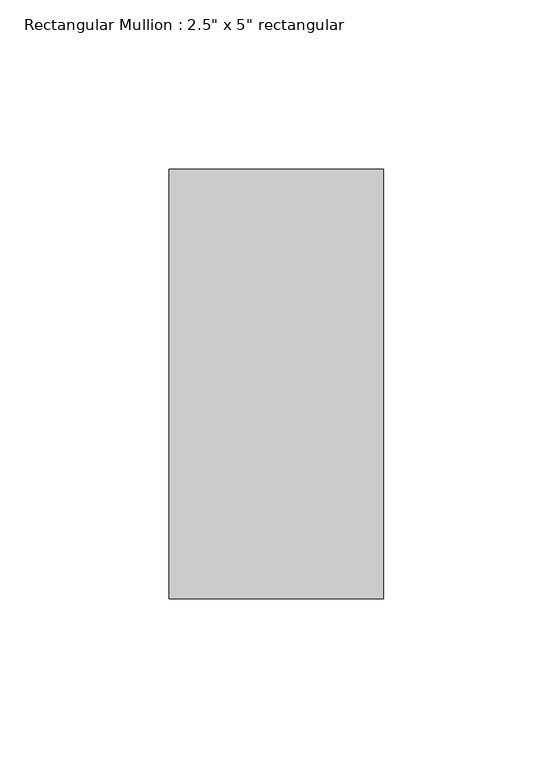
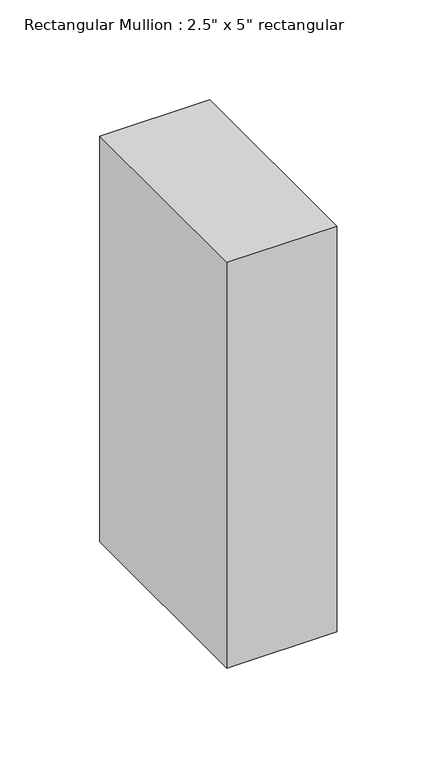
"""IFC4 building model written with IfcOpenShell, lengths in millimetres: member geometry."""

from ifc_helpers import new_model, si_unit, frame, origin, place, context, project, spatial, polyline, outline, extrude, source, transform, mapped, element, save


def member_4d06fd9b(model_context):
    return source(origin(), model_context, "Body", "SweptSolid", [
        extrude(outline(polyline([(0.0, 63.5), (0.0, -63.5), (-63.5, -63.5), (-63.5, 63.5), (0.0, 63.5)])), frame((0.0, 0.0, -247.65), z_axis=(0.0, 0.0, 1.0), x_axis=(1.0, 0.0, 0.0)), (0.0, 0.0, 1.0), 247.65),
    ])


if __name__ == "__main__":
    model = new_model("IFC4")
    model_context = context("Model", 3, world=origin())
    ifc_project = project(units=[si_unit("LENGTHUNIT", "METRE", prefix="MILLI")], contexts=[model_context])
    site = spatial("IfcSite", under=ifc_project)
    building = spatial("IfcBuilding", under=site)
    placement = place(None, origin())
    member_shape = member_4d06fd9b(model_context)
    element("IfcMember", 1, ObjectType="Rectangular Mullion : 2.5\" x 5\" rectangular", at=placement, inside=building, context=model_context, shape_type="MappedRepresentation", body=[
        mapped(member_shape, transform((0.0, 0.0, 0.0), x_axis=(1.0, 0.0, 0.0), y_axis=(0.0, 1.0, 0.0), z_axis=(0.0, 0.0, 1.0))),
    ])
    save(model, "model.ifc")

# Revit data of these elements
# Type "Rectangular Mullion : 2.5\" x 5\" rectangular"
#   built-in parameter 1007304 = 0.416667 (stored number, unit not read)
#   built-in parameter 1007301 = 0.104167 (stored number, unit not read)
#   built-in parameter 1007300 = 0.104167 (stored number, unit not read)
# Element 1 (IfcMember, "Rectangular Mullion : 2.5\" x 5\" rectangular")
#   Materials on its faces: "Aluminum"
# Materials
#   "Aluminum": class "Metal", colour RGB 247 247 247, transparency 0, Description = "Aluminum 6061", Cost = 0
